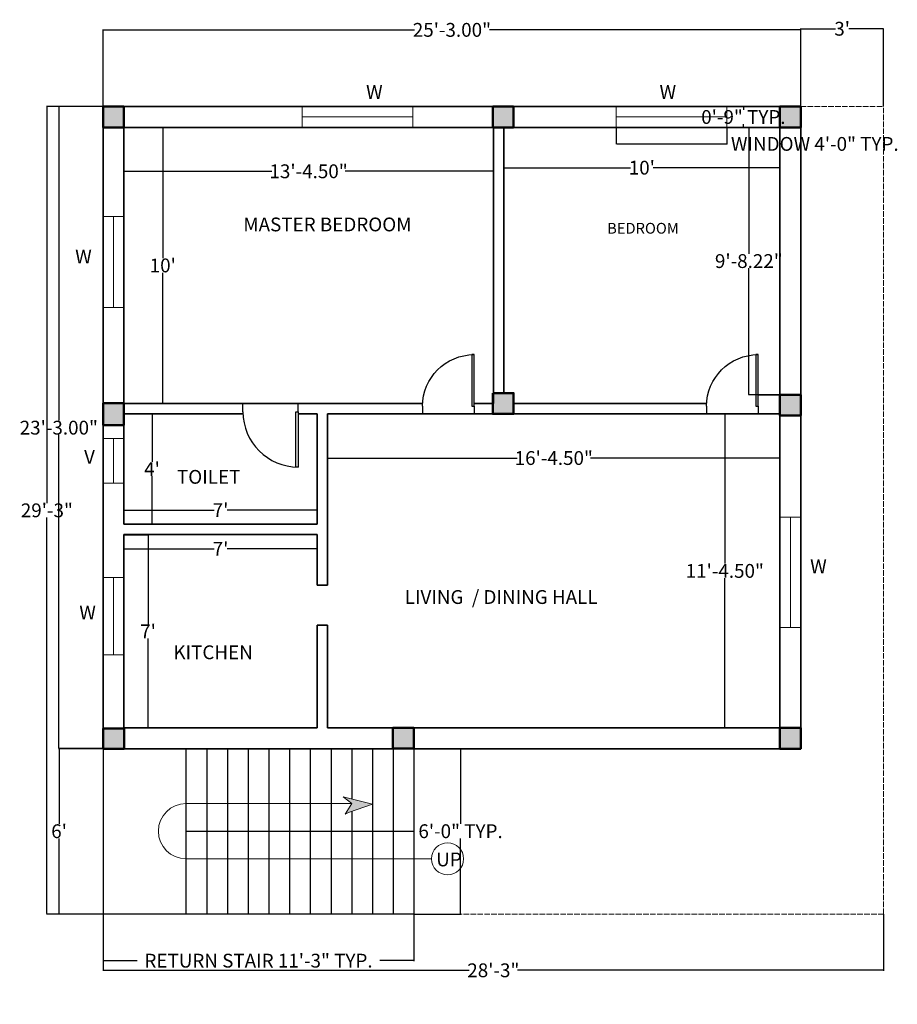
# Model space of a CAD drawing. Units: inches. Extents: x -21 to 896, y -151 to 366.
# Tile 1 of 2: x -21 to 360, y -89 to 339. Entities that reach past the tile are written whole.
import ezdxf

# ---------------------------------------------------------------- set-up
doc = ezdxf.new("R2010")
doc.units = ezdxf.units.IN
doc.header["$MEASUREMENT"] = 0
doc.linetypes.add('ACAD_ISO02W100', pattern=[15, 12, -3])
for name, color, linetype, lineweight in [('A-ANNO-DIMS', 2, 'Continuous', 18), ('A-ANNO-SYMB', 7, 'Continuous', 18), ('A-ANNO-TEXT', 7, 'Continuous', 18), ('A-AREA-IDEN', 7, 'Continuous', 25), ('A-COLS', 7, 'Continuous', 50), ('A-DOOR', 3, 'Continuous', 25), ('A-FLOR-STRS', 7, 'Continuous', 25), ('A-GLAZ', 4, 'Continuous', 18), ('A-WALL', 7, 'Continuous', 35), ('C-PROP', 8, 'ACAD_ISO02W100', 18)]:
    doc.layers.add(name, color=color, linetype=linetype, lineweight=lineweight)
doc.layers.add('A-COLS-PATT', color=18, linetype='Continuous', lineweight=13, true_color=0x000000)
doc.styles.get("Standard").update_dxf_attribs({"font": 'arial.ttf'})
doc.dimstyles.get("Standard").update_dxf_attribs({"dimtxt": 6, "dimasz": 0.18, "dimexe": 0.18, "dimexo": 0.0625, "dimgap": 0.09, "dimtad": 0, "dimtih": 1, "dimtoh": 1, "dimzin": 0, "dimdsep": 46, "dimlunit": 3, "dimtxsty": 'Standard', "dimcen": 0.09, "dimadec": 0, "dimazin": 0, "dimtfac": 1, "dimtofl": 0, "dimtmove": 0, "dimatfit": 3, "dimfxl": 1, "dimtolj": 1, "dimtzin": 0, "dimarcsym": 0})

# ---------------------------------------------------------------- blocks, each defined once
blk = doc.blocks.new('*U2')
for p, q in [((0, 0), (0, -6)), ((40, 0), (40, -6))]:
    blk.add_line(p, q)
blk.add_lwpolyline([(0, 0), (0, 40), (1.75, 40), (1.75, 0)], close=True)
blk.add_arc((0, 0), 40, 0, 90)
blk = doc.blocks.new('*D3')
at = {"layer": 'A-ANNO-DIMS', "color": 0, "lineweight": -2, "ltscale": 0.4, "transparency": 16777216}
for p, q in [((15.16, 300.94), (15.16, 334.41)), ((15.34, 334.23), (150.39, 334.23)), ((317.98, 334.23), (182.93, 334.23)), ((318.16, 300.94), (318.16, 334.41))]:
    blk.add_line(p, q, dxfattribs=at)
at = {"layer": 'A-ANNO-DIMS', "color": 0, "ltscale": 0.4, "transparency": 16777216}
for points in [[(15.34, 334.26), (15.34, 334.2), (15.16, 334.23)], [(317.98, 334.26), (317.98, 334.2), (318.16, 334.23)]]:
    blk.add_solid(points, dxfattribs=at)
at = {"layer": 'Defpoints', "color": 0, "ltscale": 0.4, "transparency": 16777216}
for p in [(318.16, 334.23), (15.16, 300.87), (318.16, 300.87)]:
    blk.add_point(p, dxfattribs=at)
at = {"layer": 'A-ANNO-DIMS', "color": 0, "ltscale": 0.4, "transparency": 16777216, "insert": (166.66, 334.23), "char_height": 6, "attachment_point": 5}
blk.add_mtext('\\A1;25\'-3.00"', dxfattribs=at)
blk = doc.blocks.new('*D4')
at = {"layer": 'A-ANNO-DIMS', "color": 0, "lineweight": -2, "ltscale": 0.4, "transparency": 16777216}
for p, q in [((24.16, 291.81), (24.16, 272.6)), ((184.66, 291.81), (184.66, 272.6)), ((24.34, 272.78), (88.47, 272.78)), ((184.48, 272.78), (120.35, 272.78))]:
    blk.add_line(p, q, dxfattribs=at)
at = {"layer": 'A-ANNO-DIMS', "color": 0, "ltscale": 0.4, "transparency": 16777216}
for points in [[(24.34, 272.81), (24.34, 272.75), (24.16, 272.78)], [(184.48, 272.81), (184.48, 272.75), (184.66, 272.78)]]:
    blk.add_solid(points, dxfattribs=at)
at = {"layer": 'Defpoints', "color": 0, "ltscale": 0.4, "transparency": 16777216}
for p in [(24.16, 291.87), (184.66, 291.87), (184.66, 272.78)]:
    blk.add_point(p, dxfattribs=at)
at = {"layer": 'A-ANNO-DIMS', "color": 0, "ltscale": 0.4, "transparency": 16777216, "insert": (104.41, 272.78), "char_height": 6, "attachment_point": 5}
blk.add_mtext('\\A1;13\'-4.50"', dxfattribs=at)
blk = doc.blocks.new('*D5')
at = {"layer": 'A-ANNO-DIMS', "color": 0, "lineweight": -2, "ltscale": 0.4, "transparency": 16777216}
for p, q in [((24.22, 291.87), (41.25, 291.87)), ((41.07, 291.69), (41.07, 235.03)), ((41.07, 172.05), (41.07, 228.72)), ((24.22, 171.87), (41.25, 171.87))]:
    blk.add_line(p, q, dxfattribs=at)
at = {"layer": 'A-ANNO-DIMS', "color": 0, "ltscale": 0.4, "transparency": 16777216}
for points in [[(41.04, 291.69), (41.1, 291.69), (41.07, 291.87)], [(41.04, 172.05), (41.1, 172.05), (41.07, 171.87)]]:
    blk.add_solid(points, dxfattribs=at)
at = {"layer": 'Defpoints', "color": 0, "ltscale": 0.4, "transparency": 16777216}
for p in [(24.16, 291.87), (41.07, 291.87), (24.16, 171.87)]:
    blk.add_point(p, dxfattribs=at)
at = {"layer": 'A-ANNO-DIMS', "color": 0, "ltscale": 0.4, "transparency": 16777216, "insert": (41.07, 231.87), "char_height": 6, "attachment_point": 5}
blk.add_mtext("\\A1;10'", dxfattribs=at)
blk = doc.blocks.new('*D6')
at = {"layer": 'A-ANNO-DIMS', "color": 0, "lineweight": -2, "ltscale": 0.4, "transparency": 16777216}
for p, q in [((189.16, 291.81), (189.16, 274.16)), ((309.16, 291.81), (309.16, 274.16)), ((189.34, 274.34), (244.26, 274.34)), ((308.98, 274.34), (254.06, 274.34))]:
    blk.add_line(p, q, dxfattribs=at)
at = {"layer": 'A-ANNO-DIMS', "color": 0, "ltscale": 0.4, "transparency": 16777216}
for points in [[(189.34, 274.37), (189.34, 274.31), (189.16, 274.34)], [(308.98, 274.37), (308.98, 274.31), (309.16, 274.34)]]:
    blk.add_solid(points, dxfattribs=at)
at = {"layer": 'Defpoints', "color": 0, "ltscale": 0.4, "transparency": 16777216}
for p in [(189.16, 291.87), (309.16, 291.87), (309.16, 274.34)]:
    blk.add_point(p, dxfattribs=at)
at = {"layer": 'A-ANNO-DIMS', "color": 0, "ltscale": 0.4, "transparency": 16777216, "insert": (249.16, 274.34), "char_height": 6, "attachment_point": 5}
blk.add_mtext("\\A1;10'", dxfattribs=at)
blk = doc.blocks.new('*D7')
at = {"layer": 'A-ANNO-DIMS', "color": 0, "lineweight": -2, "ltscale": 0.4, "transparency": 16777216}
for p, q in [((309.1, 291.87), (295.45, 291.87)), ((295.63, 291.69), (295.63, 236.92)), ((295.63, 175.83), (295.63, 230.61)), ((309.1, 175.65), (295.45, 175.65))]:
    blk.add_line(p, q, dxfattribs=at)
at = {"layer": 'A-ANNO-DIMS', "color": 0, "ltscale": 0.4, "transparency": 16777216}
for points in [[(295.6, 291.69), (295.66, 291.69), (295.63, 291.87)], [(295.6, 175.83), (295.66, 175.83), (295.63, 175.65)]]:
    blk.add_solid(points, dxfattribs=at)
at = {"layer": 'Defpoints', "color": 0, "ltscale": 0.4, "transparency": 16777216}
for p in [(295.63, 291.87), (309.16, 291.87), (309.16, 175.65)]:
    blk.add_point(p, dxfattribs=at)
at = {"layer": 'A-ANNO-DIMS', "color": 0, "ltscale": 0.4, "transparency": 16777216, "insert": (295.63, 233.76), "char_height": 6, "attachment_point": 5}
blk.add_mtext('\\A1;9\'-8.22"', dxfattribs=at)
blk = doc.blocks.new('*D8')
at = {"layer": 'A-ANNO-DIMS', "color": 0, "lineweight": -2, "ltscale": 0.4, "transparency": 16777216}
for p, q in [((15.1, 300.87), (-4.26, 300.87)), ((-4.08, 300.69), (-4.08, 164.53)), ((-4.08, 22.05), (-4.08, 158.22)), ((15.1, 21.87), (-4.26, 21.87))]:
    blk.add_line(p, q, dxfattribs=at)
at = {"layer": 'A-ANNO-DIMS', "color": 0, "ltscale": 0.4, "transparency": 16777216}
for points in [[(-4.11, 300.69), (-4.05, 300.69), (-4.08, 300.87)], [(-4.11, 22.05), (-4.05, 22.05), (-4.08, 21.87)]]:
    blk.add_solid(points, dxfattribs=at)
at = {"layer": 'Defpoints', "color": 0, "ltscale": 0.4, "transparency": 16777216}
for p in [(15.16, 300.87), (-4.08, 21.87), (15.16, 21.87)]:
    blk.add_point(p, dxfattribs=at)
at = {"layer": 'A-ANNO-DIMS', "color": 0, "ltscale": 0.4, "transparency": 16777216, "insert": (-4.08, 161.37), "char_height": 6, "attachment_point": 5}
blk.add_mtext('\\A1;23\'-3.00"', dxfattribs=at)
blk = doc.blocks.new('*D9')
at = {"layer": 'A-ANNO-DIMS', "color": 0, "lineweight": -2, "ltscale": 0.4, "transparency": 16777216}
for p, q in [((24.22, 167.37), (36.58, 167.37)), ((36.4, 167.19), (36.4, 146.46)), ((36.4, 119.55), (36.4, 140.28)), ((24.22, 119.37), (36.58, 119.37))]:
    blk.add_line(p, q, dxfattribs=at)
at = {"layer": 'A-ANNO-DIMS', "color": 0, "ltscale": 0.4, "transparency": 16777216}
for points in [[(36.37, 167.19), (36.43, 167.19), (36.4, 167.37)], [(36.37, 119.55), (36.43, 119.55), (36.4, 119.37)]]:
    blk.add_solid(points, dxfattribs=at)
at = {"layer": 'Defpoints', "color": 0, "ltscale": 0.4, "transparency": 16777216}
for p in [(24.16, 167.37), (24.16, 119.37), (36.4, 119.37)]:
    blk.add_point(p, dxfattribs=at)
at = {"layer": 'A-ANNO-DIMS', "color": 0, "ltscale": 0.4, "transparency": 16777216, "insert": (36.4, 143.37), "char_height": 6, "attachment_point": 5}
blk.add_mtext("\\A1;4'", dxfattribs=at)
blk = doc.blocks.new('*D10')
at = {"layer": 'A-ANNO-DIMS', "color": 0, "lineweight": -2, "ltscale": 0.4, "transparency": 16777216}
for p, q in [((24.16, 119.44), (24.16, 125.73)), ((24.34, 125.55), (63.33, 125.55)), ((107.98, 125.55), (68.99, 125.55)), ((108.16, 119.44), (108.16, 125.73))]:
    blk.add_line(p, q, dxfattribs=at)
at = {"layer": 'A-ANNO-DIMS', "color": 0, "ltscale": 0.4, "transparency": 16777216}
for points in [[(24.34, 125.58), (24.34, 125.52), (24.16, 125.55)], [(107.98, 125.58), (107.98, 125.52), (108.16, 125.55)]]:
    blk.add_solid(points, dxfattribs=at)
at = {"layer": 'Defpoints', "color": 0, "ltscale": 0.4, "transparency": 16777216}
for p in [(108.16, 125.55), (24.16, 119.37), (108.16, 119.37)]:
    blk.add_point(p, dxfattribs=at)
at = {"layer": 'A-ANNO-DIMS', "color": 0, "ltscale": 0.4, "transparency": 16777216, "insert": (66.16, 125.55), "char_height": 6, "attachment_point": 5}
blk.add_mtext("\\A1;7'", dxfattribs=at)
blk = doc.blocks.new('*D11')
at = {"layer": 'A-ANNO-DIMS', "color": 0, "lineweight": -2, "ltscale": 0.4, "transparency": 16777216}
for p, q in [((24.16, 114.81), (24.16, 108.52)), ((108.16, 114.81), (108.16, 108.52)), ((24.34, 108.7), (63.33, 108.7)), ((107.98, 108.7), (68.99, 108.7))]:
    blk.add_line(p, q, dxfattribs=at)
at = {"layer": 'A-ANNO-DIMS', "color": 0, "ltscale": 0.4, "transparency": 16777216}
for points in [[(24.34, 108.73), (24.34, 108.67), (24.16, 108.7)], [(107.98, 108.73), (107.98, 108.67), (108.16, 108.7)]]:
    blk.add_solid(points, dxfattribs=at)
at = {"layer": 'Defpoints', "color": 0, "ltscale": 0.4, "transparency": 16777216}
for p in [(24.16, 114.87), (108.16, 114.87), (108.16, 108.7)]:
    blk.add_point(p, dxfattribs=at)
at = {"layer": 'A-ANNO-DIMS', "color": 0, "ltscale": 0.4, "transparency": 16777216, "insert": (66.16, 108.7), "char_height": 6, "attachment_point": 5}
blk.add_mtext("\\A1;7'", dxfattribs=at)
blk = doc.blocks.new('*D12')
at = {"layer": 'A-ANNO-DIMS', "color": 0, "lineweight": -2, "ltscale": 0.4, "transparency": 16777216}
for p, q in [((24.22, 114.87), (34.86, 114.87)), ((34.68, 114.69), (34.68, 75.96)), ((34.68, 31.05), (34.68, 69.78)), ((24.22, 30.87), (34.86, 30.87))]:
    blk.add_line(p, q, dxfattribs=at)
at = {"layer": 'A-ANNO-DIMS', "color": 0, "ltscale": 0.4, "transparency": 16777216}
for points in [[(34.65, 114.69), (34.71, 114.69), (34.68, 114.87)], [(34.65, 31.05), (34.71, 31.05), (34.68, 30.87)]]:
    blk.add_solid(points, dxfattribs=at)
at = {"layer": 'Defpoints', "color": 0, "ltscale": 0.4, "transparency": 16777216}
for p in [(24.16, 114.87), (34.68, 114.87), (24.16, 30.87)]:
    blk.add_point(p, dxfattribs=at)
at = {"layer": 'A-ANNO-DIMS', "color": 0, "ltscale": 0.4, "transparency": 16777216, "insert": (34.68, 72.87), "char_height": 6, "attachment_point": 5}
blk.add_mtext("\\A1;7'", dxfattribs=at)
blk = doc.blocks.new('*D13')
at = {"layer": 'A-ANNO-DIMS', "color": 0, "lineweight": -2, "ltscale": 0.4, "transparency": 16777216}
for p, q in [((112.66, 167.31), (112.66, 147.99)), ((309.16, 167.31), (309.16, 147.99)), ((112.84, 148.17), (194.97, 148.17)), ((308.98, 148.17), (226.85, 148.17))]:
    blk.add_line(p, q, dxfattribs=at)
at = {"layer": 'A-ANNO-DIMS', "color": 0, "ltscale": 0.4, "transparency": 16777216}
for points in [[(112.84, 148.2), (112.84, 148.14), (112.66, 148.17)], [(308.98, 148.2), (308.98, 148.14), (309.16, 148.17)]]:
    blk.add_solid(points, dxfattribs=at)
at = {"layer": 'Defpoints', "color": 0, "ltscale": 0.4, "transparency": 16777216}
for p in [(112.66, 167.37), (309.16, 167.37), (309.16, 148.17)]:
    blk.add_point(p, dxfattribs=at)
at = {"layer": 'A-ANNO-DIMS', "color": 0, "ltscale": 0.4, "transparency": 16777216, "insert": (210.91, 148.17), "char_height": 6, "attachment_point": 5}
blk.add_mtext('\\A1;16\'-4.50"', dxfattribs=at)
blk = doc.blocks.new('*D14')
at = {"layer": 'A-ANNO-DIMS', "color": 0, "lineweight": -2, "ltscale": 0.4, "transparency": 16777216}
for p, q in [((309.1, 167.37), (285.01, 167.37)), ((285.19, 167.19), (285.19, 102.28)), ((285.19, 31.05), (285.19, 95.97)), ((309.1, 30.87), (285.01, 30.87))]:
    blk.add_line(p, q, dxfattribs=at)
at = {"layer": 'A-ANNO-DIMS', "color": 0, "ltscale": 0.4, "transparency": 16777216}
for points in [[(285.16, 167.19), (285.22, 167.19), (285.19, 167.37)], [(285.16, 31.05), (285.22, 31.05), (285.19, 30.87)]]:
    blk.add_solid(points, dxfattribs=at)
at = {"layer": 'Defpoints', "color": 0, "ltscale": 0.4, "transparency": 16777216}
for p in [(285.19, 167.37), (309.16, 167.37), (309.16, 30.87)]:
    blk.add_point(p, dxfattribs=at)
at = {"layer": 'A-ANNO-DIMS', "color": 0, "ltscale": 0.4, "transparency": 16777216, "insert": (285.19, 99.12), "char_height": 6, "attachment_point": 5}
blk.add_mtext('\\A1;11\'-4.50"', dxfattribs=at)
blk = doc.blocks.new('*D15')
at = {"layer": 'A-ANNO-DIMS', "color": 0, "lineweight": -2, "ltscale": 0.4, "transparency": 16777216}
for p, q in [((318.16, 300.94), (318.16, 334.89)), ((318.34, 334.71), (333.31, 334.71)), ((353.98, 334.71), (339.01, 334.71)), ((354.16, 300.94), (354.16, 334.89))]:
    blk.add_line(p, q, dxfattribs=at)
at = {"layer": 'A-ANNO-DIMS', "color": 0, "ltscale": 0.4, "transparency": 16777216}
for points in [[(318.34, 334.74), (318.34, 334.68), (318.16, 334.71)], [(353.98, 334.74), (353.98, 334.68), (354.16, 334.71)]]:
    blk.add_solid(points, dxfattribs=at)
at = {"layer": 'Defpoints', "color": 0, "ltscale": 0.4, "transparency": 16777216}
for p in [(354.16, 334.71), (318.16, 300.87), (354.16, 300.87)]:
    blk.add_point(p, dxfattribs=at)
at = {"layer": 'A-ANNO-DIMS', "color": 0, "ltscale": 0.4, "transparency": 16777216, "insert": (336.16, 334.71), "char_height": 6, "attachment_point": 5}
blk.add_mtext("\\A1;3'", dxfattribs=at)
blk = doc.blocks.new('*D16')
at = {"layer": 'A-ANNO-DIMS', "color": 0, "lineweight": -2, "ltscale": 0.4, "transparency": 16777216}
for p, q in [((15.1, 22.01), (-4.15, 22.01)), ((-3.97, 21.83), (-3.97, -10.84)), ((-3.97, -49.81), (-3.97, -17.14)), ((15.1, -49.99), (-4.15, -49.99))]:
    blk.add_line(p, q, dxfattribs=at)
at = {"layer": 'A-ANNO-DIMS', "color": 0, "ltscale": 0.4, "transparency": 16777216}
for points in [[(-4, 21.83), (-3.94, 21.83), (-3.97, 22.01)], [(-4, -49.81), (-3.94, -49.81), (-3.97, -49.99)]]:
    blk.add_solid(points, dxfattribs=at)
at = {"layer": 'Defpoints', "color": 0, "ltscale": 0.4, "transparency": 16777216}
for p in [(15.16, 22.01), (-3.97, -49.99), (15.16, -49.99)]:
    blk.add_point(p, dxfattribs=at)
at = {"layer": 'A-ANNO-DIMS', "color": 0, "ltscale": 0.4, "transparency": 16777216, "insert": (-3.97, -13.99), "char_height": 6, "attachment_point": 5}
blk.add_mtext("\\A1;6'", dxfattribs=at)
blk = doc.blocks.new('STAIR-RETURN-72IN')
for p, q in [((0, 72), (0, 0)), ((36, 72), (36, 0)), ((45, 72), (45, 0)), ((54, 72), (54, 0)), ((63, 72), (63, 0)), ((72, 72), (72, 0)), ((81, 72), (81, 0)), ((90, 72), (90, 0)), ((99, 72), (99, 0)), ((108, 72), (108, 50.05)), ((117, 72), (117, 0)), ((126, 72), (126, 0)), ((135, 72), (135, 0)), ((108, 44.67), (108, 0)), ((36, 36), (135, 36))]:
    blk.add_line(p, q)
blk.add_lwpolyline([(135, 0), (0, 0)])
blk = doc.blocks.new('STAIR-TRAVEL-UP')
h = blk.add_hatch(color=256)
h.dxf.hatch_style = 1
h.paths.add_polyline_path([(-32.62, 23.79), (-45.42, 26.99), (-41.62, 24), (-44.5, 19.46), (-43.01, 20.19)])
for p, q in [((-41.62, 24), (-45.42, 26.99)), ((-45.42, 26.99), (-32.62, 23.79)), ((-113.62, 24), (-41.62, 24)), ((-44.5, 19.46), (-41.62, 24)), ((-32.62, 23.79), (-43.01, 20.19)), ((-43.01, 20.19), (-44.5, 19.46)), ((-113.62, 0), (-14.62, 0)), ((-14.62, 0), (-6.96, 0))]:
    blk.add_line(p, q)
blk.add_circle((0, 0), 6.96)
blk.add_arc((-113.62, 12), 12, 90, 270)
at = {"insert": (-4.95, 2.74), "char_height": 6, "attachment_point": 1}
blk.add_mtext_dynamic_manual_height_columns('UP', width=3.031, gutter_width=1, heights=[0.203], dxfattribs=at)
blk = doc.blocks.new('WIN-48IN')
at = {"ltscale": 0.4}
for p, q in [((0, 9), (0, 0)), ((48, 9), (48, 0)), ((0, 4.5), (48, 4.5))]:
    blk.add_line(p, q, dxfattribs=at)
blk = doc.blocks.new('*D25')
at = {"layer": 'A-ANNO-DIMS', "color": 0, "lineweight": -2, "ltscale": 0.4, "transparency": 16777216}
for p, q in [((238.06, 291.81), (238.06, 284.49)), ((286.06, 291.81), (286.06, 284.49)), ((238.24, 284.67), (285.88, 284.67)), ((286.06, 284.67), (286.24, 284.67))]:
    blk.add_line(p, q, dxfattribs=at)
at = {"layer": 'A-ANNO-DIMS', "color": 0, "ltscale": 0.4, "transparency": 16777216}
for points in [[(238.24, 284.7), (238.24, 284.64), (238.06, 284.67)], [(285.88, 284.7), (285.88, 284.64), (286.06, 284.67)]]:
    blk.add_solid(points, dxfattribs=at)
at = {"layer": 'Defpoints', "color": 0, "ltscale": 0.4, "transparency": 16777216}
for p in [(238.06, 291.87), (286.06, 291.87), (286.06, 284.67)]:
    blk.add_point(p, dxfattribs=at)
at = {"layer": 'A-ANNO-DIMS', "color": 0, "ltscale": 0.4, "transparency": 16777216, "insert": (324.29, 284.67), "char_height": 6, "attachment_point": 5}
blk.add_mtext('\\A1;WINDOW 4\'-0" TYP.', dxfattribs=at)
blk = doc.blocks.new('*D26')
at = {"layer": 'A-ANNO-DIMS', "color": 0, "lineweight": -2, "ltscale": 0.4, "transparency": 16777216}
for p, q in [((286.12, 300.87), (293.44, 300.87)), ((293.26, 300.69), (293.26, 299.53)), ((286.12, 291.87), (293.44, 291.87)), ((293.26, 292.05), (293.26, 293.22))]:
    blk.add_line(p, q, dxfattribs=at)
at = {"layer": 'A-ANNO-DIMS', "color": 0, "ltscale": 0.4, "transparency": 16777216}
for points in [[(293.23, 300.69), (293.29, 300.69), (293.26, 300.87)], [(293.23, 292.05), (293.29, 292.05), (293.26, 291.87)]]:
    blk.add_solid(points, dxfattribs=at)
at = {"layer": 'Defpoints', "color": 0, "ltscale": 0.4, "transparency": 16777216}
for p in [(286.06, 300.87), (293.26, 300.87), (286.06, 291.87)]:
    blk.add_point(p, dxfattribs=at)
at = {"layer": 'A-ANNO-DIMS', "color": 0, "ltscale": 0.4, "transparency": 16777216, "insert": (293.26, 296.37), "char_height": 6, "attachment_point": 5}
blk.add_mtext('\\A1;0\'-9" TYP.', dxfattribs=at)
blk = doc.blocks.new('*D29')
at = {"layer": 'A-ANNO-DIMS', "color": 0, "lineweight": -2, "ltscale": 0.4, "transparency": 16777216}
for p, q in [((15.16, -50.05), (15.16, -70.42)), ((150.16, -50.05), (150.16, -70.42)), ((15.34, -70.24), (29.98, -70.24)), ((149.98, -70.24), (135.34, -70.24))]:
    blk.add_line(p, q, dxfattribs=at)
at = {"layer": 'A-ANNO-DIMS', "color": 0, "ltscale": 0.4, "transparency": 16777216}
for points in [[(15.34, -70.21), (15.34, -70.27), (15.16, -70.24)], [(149.98, -70.21), (149.98, -70.27), (150.16, -70.24)]]:
    blk.add_solid(points, dxfattribs=at)
at = {"layer": 'Defpoints', "color": 0, "ltscale": 0.4, "transparency": 16777216}
for p in [(15.16, -49.99), (150.16, -49.99), (150.16, -70.24)]:
    blk.add_point(p, dxfattribs=at)
at = {"layer": 'A-ANNO-DIMS', "color": 0, "ltscale": 0.4, "transparency": 16777216, "insert": (82.66, -70.24), "char_height": 6, "attachment_point": 5}
blk.add_mtext('\\A1;RETURN STAIR 11\'-3" TYP.', dxfattribs=at)
blk = doc.blocks.new('*D30')
at = {"layer": 'A-ANNO-DIMS', "color": 0, "lineweight": -2, "ltscale": 0.4, "transparency": 16777216}
for p, q in [((150.22, 22.01), (170.59, 22.01)), ((170.41, 21.83), (170.41, -10.84)), ((170.41, -49.81), (170.41, -17.14)), ((150.22, -49.99), (170.59, -49.99))]:
    blk.add_line(p, q, dxfattribs=at)
at = {"layer": 'A-ANNO-DIMS', "color": 0, "ltscale": 0.4, "transparency": 16777216}
for points in [[(170.38, 21.83), (170.44, 21.83), (170.41, 22.01)], [(170.38, -49.81), (170.44, -49.81), (170.41, -49.99)]]:
    blk.add_solid(points, dxfattribs=at)
at = {"layer": 'Defpoints', "color": 0, "ltscale": 0.4, "transparency": 16777216}
for p in [(150.16, 22.01), (170.41, 22.01), (150.16, -49.99)]:
    blk.add_point(p, dxfattribs=at)
at = {"layer": 'A-ANNO-DIMS', "color": 0, "ltscale": 0.4, "transparency": 16777216, "insert": (170.41, -13.99), "char_height": 6, "attachment_point": 5}
blk.add_mtext('\\A1;6\'-0" TYP.', dxfattribs=at)
blk = doc.blocks.new('*D31')
at = {"layer": 'A-ANNO-DIMS', "color": 0, "lineweight": -2, "ltscale": 0.4, "transparency": 16777216}
for p, q in [((15.1, 300.87), (-9.46, 300.87)), ((-9.28, 300.69), (-9.28, 128.6)), ((-9.28, -49.81), (-9.28, 122.29)), ((15.1, -49.99), (-9.46, -49.99))]:
    blk.add_line(p, q, dxfattribs=at)
at = {"layer": 'A-ANNO-DIMS', "color": 0, "ltscale": 0.4, "transparency": 16777216}
for points in [[(-9.31, 300.69), (-9.25, 300.69), (-9.28, 300.87)], [(-9.31, -49.81), (-9.25, -49.81), (-9.28, -49.99)]]:
    blk.add_solid(points, dxfattribs=at)
at = {"layer": 'Defpoints', "color": 0, "ltscale": 0.4, "transparency": 16777216}
for p in [(-9.28, 300.87), (15.16, 300.87), (15.16, -49.99)]:
    blk.add_point(p, dxfattribs=at)
at = {"layer": 'A-ANNO-DIMS', "color": 0, "ltscale": 0.4, "transparency": 16777216, "insert": (-9.28, 125.44), "char_height": 6, "attachment_point": 5}
blk.add_mtext('\\A1;29\'-3"', dxfattribs=at)
blk = doc.blocks.new('*D32')
at = {"layer": 'A-ANNO-DIMS', "color": 0, "lineweight": -2, "ltscale": 0.4, "transparency": 16777216}
for p, q in [((15.16, -50.05), (15.16, -74.61)), ((354.16, -50.05), (354.16, -74.61)), ((15.34, -74.43), (174.21, -74.43)), ((353.98, -74.43), (195.11, -74.43))]:
    blk.add_line(p, q, dxfattribs=at)
at = {"layer": 'A-ANNO-DIMS', "color": 0, "ltscale": 0.4, "transparency": 16777216}
for points in [[(15.34, -74.4), (15.34, -74.46), (15.16, -74.43)], [(353.98, -74.4), (353.98, -74.46), (354.16, -74.43)]]:
    blk.add_solid(points, dxfattribs=at)
at = {"layer": 'Defpoints', "color": 0, "ltscale": 0.4, "transparency": 16777216}
for p in [(15.16, -49.99), (354.16, -49.99), (354.16, -74.43)]:
    blk.add_point(p, dxfattribs=at)
at = {"layer": 'A-ANNO-DIMS', "color": 0, "ltscale": 0.4, "transparency": 16777216, "insert": (184.66, -74.43), "char_height": 6, "attachment_point": 5}
blk.add_mtext('\\A1;28\'-3"', dxfattribs=at)

msp = doc.modelspace()

# ---------------------------------------------------------------- hatches: boundary and pattern name
at = {"layer": 'A-COLS-PATT', "ltscale": 0.4}
h = msp.add_hatch(color=256, dxfattribs=at)
h.dxf.hatch_style = 1
h.paths.add_polyline_path([(24.159, 291.873), (24.159, 300.873), (15.159, 300.873), (15.159, 291.873)])
h.paths.add_polyline_path([(24.339, 21.873), (24.339, 30.653), (15.159, 30.653), (15.159, 21.873)])
h.paths.add_polyline_path([(150.159, 30.873), (140.939, 30.873), (140.939, 22.008), (150.159, 22.008)])
h.paths.add_polyline_path([(309.159, 30.873), (309.159, 21.873), (318.159, 21.873), (318.159, 30.873)])
h = msp.add_hatch(color=256, dxfattribs=at)
h.dxf.hatch_style = 1
h.paths.add_polyline_path([(193.429, 176.373), (184.659, 176.373), (184.659, 171.873), (184.429, 171.873), (184.429, 167.373), (193.429, 167.373)])
h.paths.add_polyline_path([(318.159, 175.65), (309.159, 175.65), (309.159, 166.65), (318.159, 166.65)])
h.paths.add_polyline_path([(318.159, 300.873), (309.159, 300.873), (309.159, 291.873), (318.159, 291.873)])
h.paths.add_polyline_path([(193.46, 300.873), (184.46, 300.873), (184.46, 291.873), (193.46, 291.873)])
h = msp.add_hatch(color=256, dxfattribs=at)
h.dxf.hatch_style = 1
h.paths.add_polyline_path([(24.159, 172.031), (15.159, 172.031), (15.159, 162.484), (24.159, 162.484)])

# ---------------------------------------------------------------- linework, layer by layer
at = {"layer": 'A-COLS', "ltscale": 0.4}
for points in [[(15.159, 300.873), (24.159, 300.873), (24.159, 291.873), (15.159, 291.873)], [(184.46, 300.873), (193.46, 300.873), (193.46, 291.873), (184.46, 291.873)], [(309.159, 300.873), (318.159, 300.873), (318.159, 291.873), (309.159, 291.873)], [(184.429, 176.373), (193.429, 176.373), (193.429, 167.373), (184.429, 167.373)], [(309.159, 175.65), (318.159, 175.65), (318.159, 166.65), (309.159, 166.65)], [(15.159, 172.031), (24.159, 172.031), (24.159, 162.484), (15.159, 162.484)], [(15.159, 30.653), (24.339, 30.653), (24.339, 21.873), (15.159, 21.873)], [(140.939, 30.873), (150.159, 30.873), (150.159, 22.008), (140.939, 22.008)], [(309.159, 30.873), (318.159, 30.873), (318.159, 21.873), (309.159, 21.873)]]:
    msp.add_lwpolyline(points, close=True, dxfattribs=at)
at = {"layer": 'A-GLAZ', "ltscale": 0.4}
for p, q in [((15.159, 253.072), (24.159, 253.072)), ((19.659, 213.636), (19.659, 253.072)), ((15.159, 213.636), (24.159, 213.636)), ((24.159, 213.636), (19.659, 213.636)), ((15.159, 156.652), (24.159, 156.652)), ((19.659, 137.293), (19.659, 156.652)), ((15.159, 137.293), (24.159, 137.293)), ((15.159, 96.237), (24.159, 96.237)), ((19.659, 62.675), (19.659, 96.237)), ((15.159, 62.675), (24.159, 62.675))]:
    msp.add_line(p, q, dxfattribs=at)
at = {"layer": 'A-WALL', "ltscale": 0.4}
for p, q in [((108.159, 92.907), (112.659, 92.907)), ((108.159, 75.525), (112.659, 75.525))]:
    msp.add_line(p, q, dxfattribs=at)
at = {"layer": 'A-WALL'}
msp.add_lwpolyline([(15.159, 21.873), (318.159, 21.873), (318.159, 300.873), (15.159, 300.873)], close=True, dxfattribs=at)
for points in [[(24.159, 291.873), (24.159, 171.873)], [(184.659, 291.873), (24.159, 291.873)], [(184.659, 291.873), (184.659, 171.873)], [(309.159, 291.873), (189.159, 291.873)], [(189.159, 176.373), (189.159, 291.873)], [(309.159, 175.65), (309.159, 291.873)], [(309.159, 175.65), (299.648, 175.65)], [(153.938, 171.873), (24.159, 171.873)], [(184.659, 171.873), (176.28, 171.873)], [(277.306, 171.873), (193.429, 171.873)], [(75.926, 167.373), (24.159, 167.373)], [(24.159, 167.373), (24.159, 119.373)], [(108.159, 167.373), (99.938, 167.373)], [(108.159, 119.373), (108.159, 167.373)], [(309.159, 167.373), (112.659, 167.373)], [(112.659, 92.907), (112.659, 167.373)], [(309.159, 30.873), (309.159, 167.373)], [(108.159, 119.373), (24.159, 119.373)], [(24.159, 114.873), (108.159, 114.873)], [(24.159, 114.873), (24.159, 30.873)], [(108.159, 92.907), (108.159, 114.873)], [(108.159, 30.873), (108.159, 75.525)], [(112.659, 30.873), (112.659, 75.525)], [(24.159, 30.873), (108.159, 30.873)], [(112.659, 30.873), (309.159, 30.873)]]:
    msp.add_lwpolyline(points, dxfattribs=at)
at = {"layer": 'C-PROP', "ltscale": 0.2}
msp.add_line((318.159, 300.873), (354.159, 300.873), dxfattribs=at)
for points in [[(354.159, -49.992), (354.159, 300.873)], [(354.159, -49.992), (150.159, -49.992)]]:
    msp.add_lwpolyline(points, dxfattribs=at)

# ---------------------------------------------------------------- block references
at = {"layer": 'A-ANNO-SYMB'}
msp.add_blockref('STAIR-TRAVEL-UP', (164.782, -25.992), dxfattribs=at)
at = {"layer": 'A-DOOR', "xscale": -0.5592774159886474, "yscale": 0.5592774159886474, "zscale": 0.5592774159886474}
for p in [(176.28, 170.729), (299.648, 170.729)]:
    msp.add_blockref('*U2', p, dxfattribs=at)
at = {"layer": 'A-DOOR', "xscale": 0.6007338957814297, "yscale": 0.6007338957814297, "zscale": 0.6007338957814297, "rotation": 180}
msp.add_blockref('*U2', (99.938, 168.269), dxfattribs=at)
at = {"layer": 'A-FLOR-STRS'}
msp.add_blockref('STAIR-RETURN-72IN', (15.159, -49.992), dxfattribs=at)
at = {"layer": 'A-GLAZ'}
for p in [(101.636, 291.873), (238.059, 291.873)]:
    msp.add_blockref('WIN-48IN', p, dxfattribs=at)
at = {"layer": 'A-GLAZ', "rotation": 269.9999999999998}
msp.add_blockref('WIN-48IN', (309.159, 122.532), dxfattribs=at)

# ---------------------------------------------------------------- texts
at = {"layer": 'A-ANNO-TEXT', "char_height": 6, "attachment_point": 1}
for s, insert in [('W', (129.38, 310.228)), ('W', (256.853, 310.228)), ('W', (3.025, 238.721)), ('V', (6.891, 151.734)), ('W', (322.267, 104.086)), ('W', (4.816, 84.04))]:
    msp.add_mtext_dynamic_manual_height_columns(s, width=6, gutter_width=1, heights=[0.203], dxfattribs=dict(at, insert=insert))
at = {"layer": 'A-AREA-IDEN', "attachment_point": 1}
for s, width, gutter_width, insert, char_height in [('MASTER BEDROOM', 173.95707, 1, (76.053, 252.677), 6), ('BEDROOM ', 135.93882, 0.781, (234.08, 250.357), 4.6887), ('TOILET', 173.95707, 1, (47.234, 142.984), 6), ('LIVING  / DINING HALL', 173.95707, 1, (146.163, 90.769), 6), ('KITCHEN ', 173.95707, 1, (45.677, 66.756), 6)]:
    msp.add_mtext_dynamic_manual_height_columns(s, width=width, gutter_width=gutter_width, heights=[0], dxfattribs=dict(at, insert=insert, char_height=char_height))

# ---------------------------------------------------------------- dimensions: what is measured, and where the dimension line sits
at = {"layer": 'A-ANNO-DIMS', "ltscale": 0.4}
for base, p1, p2, override, picture, middle in [((318.159, 334.233), (15.159, 300.873), (318.159, 300.873), {"dimclrd": 0, "dimclre": 0, "dimclrt": 0}, '*D3', (166.659, 334.233)), ((354.159, 334.713), (318.159, 300.873), (354.159, 300.873), {"dimclrd": 0, "dimclre": 0, "dimclrt": 0}, '*D15', (336.159, 334.713)), ((184.659, 272.784), (24.159, 291.873), (184.659, 291.873), {"dimclrd": 0, "dimclre": 0, "dimclrt": 0}, '*D4', (104.409, 272.784)), ((309.159, 274.339), (189.159, 291.873), (309.159, 291.873), {"dimclrd": 0, "dimclre": 0, "dimclrt": 0}, '*D6', (249.159, 274.339)), ((309.159, 148.168), (112.659, 167.373), (309.159, 167.373), {"dimclrd": 0, "dimclre": 0, "dimclrt": 0}, '*D13', (210.909, 148.168)), ((108.159, 125.555), (24.159, 119.373), (108.159, 119.373), {"dimclrd": 0, "dimclre": 0, "dimclrt": 0}, '*D10', (66.159, 125.555)), ((108.159, 108.698), (24.159, 114.873), (108.159, 114.873), {"dimclrd": 0, "dimclre": 0, "dimclrt": 0}, '*D11', (66.159, 108.698)), ((354.159, -74.432), (15.159, -49.992), (354.159, -49.992), {"dimdec": 1, "dimlfac": 1, "dimrnd": 0, "dimzin": 1, "dimdsep": 46, "dimlunit": 4, "dimfrac": 2}, '*D32', (184.659, -74.432))]:
    dim = msp.add_linear_dim(base=base, p1=p1, p2=p2, dimstyle='Standard', override=override, dxfattribs=at)
    dim.commit()
    dim.dimension.update_dxf_attribs({"geometry": picture, "text_midpoint": middle})
for base, p1, p2, picture, middle in [((293.259, 300.873), (286.059, 291.873), (286.059, 300.873), '*D26', (293.259, 296.373)), ((170.409, 22.008), (150.159, -49.992), (150.159, 22.008), '*D30', (170.409, -13.992))]:
    dim = msp.add_linear_dim(base=base, p1=p1, p2=p2, angle=90, text='<> TYP.', dimstyle='Standard', override={"dimdec": 1, "dimlfac": 1, "dimrnd": 0, "dimzin": 1, "dimdsep": 46, "dimlunit": 4, "dimfrac": 2}, dxfattribs=at)
    dim.commit()
    dim.dimension.update_dxf_attribs({"geometry": picture, "text_midpoint": middle})
for base, p1, p2, override, picture, middle in [((-4.08, 21.873), (15.159, 300.873), (15.159, 21.873), {"dimclrd": 0, "dimclre": 0, "dimclrt": 0}, '*D8', (-4.08, 161.373)), ((-9.281, 300.873), (15.159, -49.992), (15.159, 300.873), {"dimdec": 1, "dimlfac": 1, "dimrnd": 0, "dimzin": 1, "dimdsep": 46, "dimlunit": 4, "dimfrac": 2}, '*D31', (-9.281, 125.441)), ((41.071, 291.873), (24.159, 171.873), (24.159, 291.873), {"dimclrd": 0, "dimclre": 0, "dimclrt": 0}, '*D5', (41.071, 231.873)), ((295.626, 291.873), (309.159, 175.65), (309.159, 291.873), {"dimclrd": 0, "dimclre": 0, "dimclrt": 0}, '*D7', (295.626, 233.762)), ((36.4, 119.373), (24.159, 167.373), (24.159, 119.373), {"dimclrd": 0, "dimclre": 0, "dimclrt": 0}, '*D9', (36.4, 143.373)), ((285.188, 167.373), (309.159, 30.873), (309.159, 167.373), {"dimclrd": 0, "dimclre": 0, "dimclrt": 0}, '*D14', (285.188, 99.123)), ((34.681, 114.873), (24.159, 30.873), (24.159, 114.873), {"dimclrd": 0, "dimclre": 0, "dimclrt": 0}, '*D12', (34.681, 72.873)), ((-3.969, -49.992), (15.159, 22.008), (15.159, -49.992), {"dimclrd": 0, "dimclre": 0, "dimclrt": 0}, '*D16', (-3.969, -13.992))]:
    dim = msp.add_linear_dim(base=base, p1=p1, p2=p2, angle=90, dimstyle='Standard', override=override, dxfattribs=at)
    dim.commit()
    dim.dimension.update_dxf_attribs({"geometry": picture, "text_midpoint": middle})
for base, p1, p2, text, picture, middle in [((286.059, 284.673), (238.059, 291.873), (286.059, 291.873), 'WINDOW <> TYP.', '*D25', (324.291, 284.673)), ((150.159, -70.242), (15.159, -49.992), (150.159, -49.992), 'RETURN STAIR <> TYP.', '*D29', (82.659, -70.242))]:
    dim = msp.add_linear_dim(base=base, p1=p1, p2=p2, text=text, dimstyle='Standard', override={"dimdec": 1, "dimlfac": 1, "dimrnd": 0, "dimzin": 1, "dimdsep": 46, "dimlunit": 4, "dimfrac": 2}, dxfattribs=at)
    dim.commit()
    dim.dimension.update_dxf_attribs({"geometry": picture, "text_midpoint": middle})

doc.saveas('drawing.dxf')
